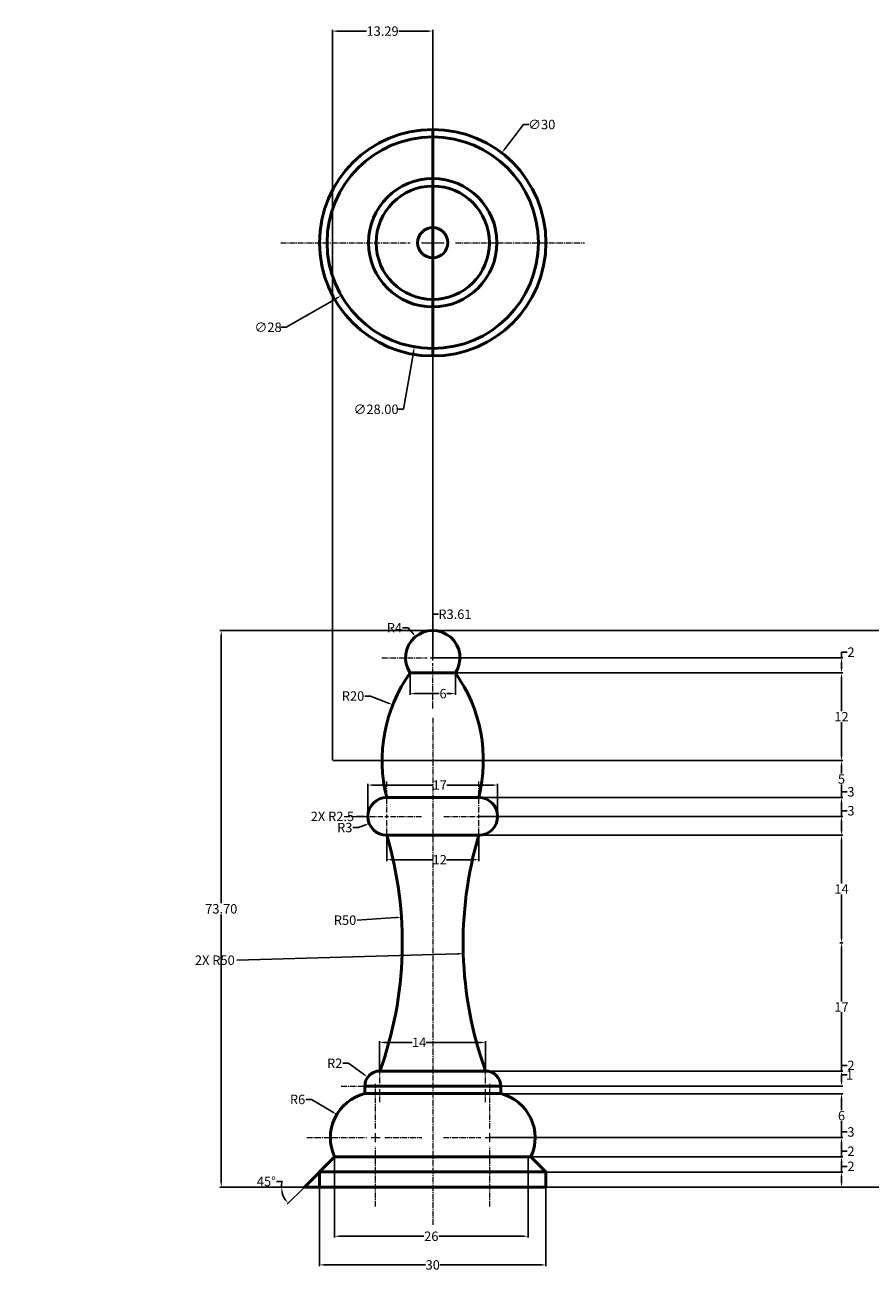
# Model space of a CAD drawing. Units: millimetres. Extents: x 184 to 390, y 95 to 263.
# Tile 1 of 2: x 184 to 296, y 98 to 263. Entities that reach past the tile are written whole.
import ezdxf

# ---------------------------------------------------------------- set-up
doc = ezdxf.new("R2010")
doc.units = ezdxf.units.MM
doc.header["$MEASUREMENT"] = 0
doc.linetypes.add('CENTER2', pattern=[1.125, 0.75, -0.125, 0.125, -0.125])
for name, color, linetype, lineweight in [('M-CNTR', 1, 'CENTER2', 18), ('M-DIMS', 2, 'Continuous', 25), ('M-OUTL', 7, 'Continuous', 50)]:
    doc.layers.add(name, color=color, linetype=linetype, lineweight=lineweight)
doc.styles.get("Standard").update_dxf_attribs({"font": 'arial.ttf'})
doc.dimstyles.get("Standard").update_dxf_attribs({"dimtxt": 1.25, "dimasz": 0.75, "dimexe": 0.18, "dimexo": 0.0625, "dimgap": 0.09, "dimtad": 0, "dimtih": 1, "dimtoh": 1, "dimdec": 0, "dimzin": 0, "dimdsep": 46, "dimtxsty": 'Standard', "dimcen": 0.09, "dimadec": 0, "dimazin": 0, "dimtfac": 1, "dimtdec": 0, "dimtofl": 0, "dimtmove": 0, "dimatfit": 3, "dimfxl": 1, "dimtolj": 1, "dimtzin": 0, "dimarcsym": 0})

# ---------------------------------------------------------------- blocks, each defined once
blk = doc.blocks.new('*D1')
at = {"layer": 'Defpoints', "color": 0, "transparency": 16777216}
for p in [(225.21, 112.98), (221.21, 108.98), (221.21, 108.98), (223.21, 108.98), (218.57, 107.46)]:
    blk.add_point(p, dxfattribs=at)
at = {"layer": 'M-DIMS', "color": 0, "lineweight": -2, "transparency": 16777216}
for p, q in [((218.26, 109.73), (217.51, 109.73)), ((221.15, 108.98), (217.99, 108.98)), ((221.16, 108.94), (218.93, 106.71))]:
    blk.add_line(p, q, dxfattribs=at)
for start, end in [(165.8396, 180), (194.1604, 210.8396)]:
    blk.add_arc((221.21, 108.98), 3.04, start, end, dxfattribs=at)
at = {"layer": 'M-DIMS', "color": 0, "transparency": 16777216}
for points in [[(218.13, 108.22), (218.38, 108.26), (218.17, 108.98)], [(218.69, 107.5), (218.5, 107.35), (219.06, 106.83)]]:
    blk.add_solid(points, dxfattribs=at)
at = {"layer": 'M-DIMS', "color": 0, "transparency": 16777216, "insert": (216.17, 109.73), "char_height": 1.25, "attachment_point": 5}
blk.add_mtext('\\A1;45°', dxfattribs=at)
blk = doc.blocks.new('*D2')
at = {"layer": 'Defpoints', "color": 0, "transparency": 16777216}
for p in [(247.35, 245.93), (229.07, 222.14)]:
    blk.add_point(p, dxfattribs=at)
at = {"layer": 'M-DIMS', "color": 0, "lineweight": -2, "transparency": 16777216}
for p, q in [((250.24, 249.69), (247.8, 246.53)), ((250.99, 249.69), (250.24, 249.69)), ((238.12, 234.04), (238.3, 234.04)), ((238.21, 233.95), (238.21, 234.13))]:
    blk.add_line(p, q, dxfattribs=at)
at = {"layer": 'M-DIMS', "color": 0, "transparency": 16777216}
blk.add_solid([(247.71, 246.6), (247.9, 246.45), (247.35, 245.93)], dxfattribs=at)
at = {"layer": 'M-DIMS', "color": 0, "transparency": 16777216, "insert": (252.65, 249.69), "char_height": 1.25, "attachment_point": 5}
blk.add_mtext('\\A1;∅30', dxfattribs=at)
blk = doc.blocks.new('*U3')
at = {"layer": 'M-CNTR', "color": 0, "transparency": 16777216}
for p, q in [((0, 3), (0, 20.12)), ((-20.12, 0), (-3, 0)), ((3, 0), (20.12, 0)), ((0, -20.12), (0, -3))]:
    blk.add_line(p, q, dxfattribs=at)
at = {"layer": 'M-CNTR', "color": 0, "linetype": 'Continuous', "transparency": 16777216}
for p, q in [((-1.5, 0), (1.5, 0)), ((0, -1.5), (0, 1.5))]:
    blk.add_line(p, q, dxfattribs=at)
blk = doc.blocks.new('*U4')
at = {"layer": 'M-CNTR', "color": 0, "transparency": 16777216}
for p, q in [((0, 0.72), (0, 8.73)), ((-6.73, 0), (-0.72, 0)), ((0.72, 0), (6.73, 0)), ((0, -6.73), (0, -0.72))]:
    blk.add_line(p, q, dxfattribs=at)
at = {"layer": 'M-CNTR', "color": 0, "linetype": 'Continuous', "transparency": 16777216}
for p, q in [((-0.36, 0), (0.36, 0)), ((0, -0.36), (0, 0.36))]:
    blk.add_line(p, q, dxfattribs=at)
blk = doc.blocks.new('*U5')
at = {"layer": 'M-CNTR', "color": 0, "transparency": 16777216}
for p, q in [((0, 0.5), (0, 4.62)), ((-5.62, 0), (-0.5, 0)), ((0.5, 0), (4.62, 0)), ((0, -4.62), (0, -0.5))]:
    blk.add_line(p, q, dxfattribs=at)
at = {"layer": 'M-CNTR', "color": 0, "linetype": 'Continuous', "transparency": 16777216}
for p, q in [((-0.25, 0), (0.25, 0)), ((0, -0.25), (0, 0.25))]:
    blk.add_line(p, q, dxfattribs=at)
blk = doc.blocks.new('*U6')
at = {"layer": 'M-CNTR', "color": 0, "transparency": 16777216}
for p, q in [((0, 0.5), (0, 4.62)), ((-4.62, 0), (-0.5, 0)), ((0.5, 0), (5.62, 0)), ((0, -4.62), (0, -0.5))]:
    blk.add_line(p, q, dxfattribs=at)
at = {"layer": 'M-CNTR', "color": 0, "linetype": 'Continuous', "transparency": 16777216}
for p, q in [((-0.25, 0), (0.25, 0)), ((0, -0.25), (0, 0.25))]:
    blk.add_line(p, q, dxfattribs=at)
blk = doc.blocks.new('*U7')
at = {"layer": 'M-CNTR', "color": 0, "transparency": 16777216}
for p, q in [((0, 1.2), (0, 7.12)), ((-9.12, 0), (-1.2, 0)), ((1.2, 0), (6.12, 0)), ((0, -9.12), (0, -1.2))]:
    blk.add_line(p, q, dxfattribs=at)
at = {"layer": 'M-CNTR', "color": 0, "linetype": 'Continuous', "transparency": 16777216}
for p, q in [((-0.6, 0), (0.6, 0)), ((0, -0.6), (0, 0.6))]:
    blk.add_line(p, q, dxfattribs=at)
blk = doc.blocks.new('*U8')
at = {"layer": 'M-CNTR', "color": 0, "transparency": 16777216}
for p, q in [((0, 1.2), (0, 7.12)), ((-6.12, 0), (-1.2, 0)), ((1.2, 0), (9.12, 0)), ((0, -9.12), (0, -1.2))]:
    blk.add_line(p, q, dxfattribs=at)
at = {"layer": 'M-CNTR', "color": 0, "linetype": 'Continuous', "transparency": 16777216}
for p, q in [((-0.6, 0), (0.6, 0)), ((0, -0.6), (0, 0.6))]:
    blk.add_line(p, q, dxfattribs=at)
blk = doc.blocks.new('*U9')
at = {"layer": 'M-CNTR', "color": 0, "transparency": 16777216}
for p, q in [((0, 0.4), (0, 4.12)), ((-2.12, 0), (-0.4, 0)), ((0.4, 0), (5.12, 0)), ((0, -2.12), (0, -0.4))]:
    blk.add_line(p, q, dxfattribs=at)
at = {"layer": 'M-CNTR', "color": 0, "linetype": 'Continuous', "transparency": 16777216}
for p, q in [((-0.2, 0), (0.2, 0)), ((0, -0.2), (0, 0.2))]:
    blk.add_line(p, q, dxfattribs=at)
blk = doc.blocks.new('*U10')
at = {"layer": 'M-CNTR', "color": 0, "transparency": 16777216}
for p, q in [((0, 0.4), (0, 4.12)), ((-5.12, 0), (-0.4, 0)), ((0.4, 0), (2.12, 0)), ((0, -2.12), (0, -0.4))]:
    blk.add_line(p, q, dxfattribs=at)
at = {"layer": 'M-CNTR', "color": 0, "linetype": 'Continuous', "transparency": 16777216}
for p, q in [((-0.2, 0), (0.2, 0)), ((0, -0.2), (0, 0.2))]:
    blk.add_line(p, q, dxfattribs=at)
blk = doc.blocks.new('*U11')
at = {"layer": 'M-CNTR', "color": 0, "transparency": 16777216}
blk.add_line((0, 61.12), (0, -6.12), dxfattribs=at)
blk = doc.blocks.new('*D12')
at = {"layer": 'Defpoints', "color": 0, "transparency": 16777216}
for p in [(235.93, 181.87), (238.21, 179.07)]:
    blk.add_point(p, dxfattribs=at)
at = {"layer": 'M-DIMS', "color": 0, "lineweight": -2, "transparency": 16777216}
for p, q in [((234.22, 183.05), (234.97, 183.05)), ((234.97, 183.05), (235.46, 182.45)), ((238.12, 179.07), (238.3, 179.07)), ((238.21, 178.98), (238.21, 179.16))]:
    blk.add_line(p, q, dxfattribs=at)
at = {"layer": 'M-DIMS', "color": 0, "transparency": 16777216}
blk.add_solid([(235.56, 182.53), (235.36, 182.38), (235.93, 181.87)], dxfattribs=at)
at = {"layer": 'M-DIMS', "color": 0, "transparency": 16777216, "insert": (233.13, 183.05), "char_height": 1.25, "attachment_point": 5}
blk.add_mtext('\\A1;R4', dxfattribs=at)
blk = doc.blocks.new('*D13')
at = {"layer": 'Defpoints', "color": 0, "transparency": 16777216}
for p in [(253.21, 110.98), (292.36, 110.98), (253.21, 108.98)]:
    blk.add_point(p, dxfattribs=at)
at = {"layer": 'M-DIMS', "color": 0, "lineweight": -2, "transparency": 16777216}
for p, q in [((253.27, 110.98), (292.54, 110.98)), ((292.36, 110.98), (292.36, 111.73)), ((292.36, 111.73), (293.11, 111.73)), ((253.27, 108.98), (292.54, 108.98)), ((292.36, 109.73), (292.36, 110.23))]:
    blk.add_line(p, q, dxfattribs=at)
at = {"layer": 'M-DIMS', "color": 0, "transparency": 16777216}
for points in [[(292.24, 110.23), (292.49, 110.23), (292.36, 110.98)], [(292.24, 109.73), (292.49, 109.73), (292.36, 108.98)]]:
    blk.add_solid(points, dxfattribs=at)
at = {"layer": 'M-DIMS', "color": 0, "transparency": 16777216, "insert": (293.62, 111.73), "char_height": 1.25, "attachment_point": 5}
blk.add_mtext('\\A1;2', dxfattribs=at)
blk = doc.blocks.new('*D14')
at = {"layer": 'Defpoints', "color": 0, "transparency": 16777216}
for p in [(251.21, 112.98), (292.36, 112.98), (253.21, 110.98)]:
    blk.add_point(p, dxfattribs=at)
at = {"layer": 'M-DIMS', "color": 0, "lineweight": -2, "transparency": 16777216}
for p, q in [((251.27, 112.98), (292.54, 112.98)), ((292.36, 112.98), (292.36, 113.73)), ((292.36, 113.73), (293.11, 113.73)), ((292.36, 111.73), (292.36, 112.23)), ((253.27, 110.98), (292.54, 110.98))]:
    blk.add_line(p, q, dxfattribs=at)
at = {"layer": 'M-DIMS', "color": 0, "transparency": 16777216}
for points in [[(292.24, 112.23), (292.49, 112.23), (292.36, 112.98)], [(292.24, 111.73), (292.49, 111.73), (292.36, 110.98)]]:
    blk.add_solid(points, dxfattribs=at)
at = {"layer": 'M-DIMS', "color": 0, "transparency": 16777216, "insert": (293.62, 113.73), "char_height": 1.25, "attachment_point": 5}
blk.add_mtext('\\A1;2', dxfattribs=at)
blk = doc.blocks.new('*D15')
at = {"layer": 'Defpoints', "color": 0, "transparency": 16777216}
for p in [(245.77, 115.53), (292.36, 115.53), (251.21, 112.98)]:
    blk.add_point(p, dxfattribs=at)
at = {"layer": 'M-DIMS', "color": 0, "lineweight": -2, "transparency": 16777216}
for p, q in [((245.84, 115.53), (292.54, 115.53)), ((292.36, 115.53), (292.36, 116.28)), ((292.36, 116.28), (293.11, 116.28)), ((292.36, 113.73), (292.36, 114.78)), ((251.27, 112.98), (292.54, 112.98))]:
    blk.add_line(p, q, dxfattribs=at)
at = {"layer": 'M-DIMS', "color": 0, "transparency": 16777216}
for points in [[(292.24, 114.78), (292.49, 114.78), (292.36, 115.53)], [(292.24, 113.73), (292.49, 113.73), (292.36, 112.98)]]:
    blk.add_solid(points, dxfattribs=at)
at = {"layer": 'M-DIMS', "color": 0, "transparency": 16777216, "insert": (293.61, 116.28), "char_height": 1.25, "attachment_point": 5}
blk.add_mtext('\\A1;3', dxfattribs=at)
blk = doc.blocks.new('*D16')
at = {"layer": 'Defpoints', "color": 0, "transparency": 16777216}
for p in [(247.21, 121.35), (292.36, 121.35), (245.77, 115.53)]:
    blk.add_point(p, dxfattribs=at)
at = {"layer": 'M-DIMS', "color": 0, "lineweight": -2, "transparency": 16777216}
for p, q in [((247.27, 121.35), (292.54, 121.35)), ((292.36, 120.6), (292.36, 119.17)), ((292.36, 116.28), (292.36, 117.71)), ((245.84, 115.53), (292.54, 115.53))]:
    blk.add_line(p, q, dxfattribs=at)
at = {"layer": 'M-DIMS', "color": 0, "transparency": 16777216}
for points in [[(292.24, 120.6), (292.49, 120.6), (292.36, 121.35)], [(292.24, 116.28), (292.49, 116.28), (292.36, 115.53)]]:
    blk.add_solid(points, dxfattribs=at)
at = {"layer": 'M-DIMS', "color": 0, "transparency": 16777216, "insert": (292.36, 118.44), "char_height": 1.25, "attachment_point": 5}
blk.add_mtext('\\A1;6', dxfattribs=at)
blk = doc.blocks.new('*D17')
at = {"layer": 'Defpoints', "color": 0, "transparency": 16777216}
for p in [(247.21, 122.35), (292.36, 122.35), (247.21, 121.35)]:
    blk.add_point(p, dxfattribs=at)
at = {"layer": 'M-DIMS', "color": 0, "lineweight": -2, "transparency": 16777216}
for p, q in [((292.36, 123.1), (292.36, 123.85)), ((292.36, 123.85), (293.11, 123.85)), ((247.27, 122.35), (292.54, 122.35)), ((247.27, 121.35), (292.54, 121.35)), ((292.36, 120.6), (292.36, 119.85))]:
    blk.add_line(p, q, dxfattribs=at)
at = {"layer": 'M-DIMS', "color": 0, "transparency": 16777216}
for points in [[(292.24, 123.1), (292.49, 123.1), (292.36, 122.35)], [(292.24, 120.6), (292.49, 120.6), (292.36, 121.35)]]:
    blk.add_solid(points, dxfattribs=at)
at = {"layer": 'M-DIMS', "color": 0, "transparency": 16777216, "insert": (293.43, 123.85), "char_height": 1.25, "attachment_point": 5}
blk.add_mtext('\\A1;1', dxfattribs=at)
blk = doc.blocks.new('*D18')
at = {"layer": 'Defpoints', "color": 0, "transparency": 16777216}
for p in [(245.21, 124.35), (292.36, 124.35), (247.21, 122.35)]:
    blk.add_point(p, dxfattribs=at)
at = {"layer": 'M-DIMS', "color": 0, "lineweight": -2, "transparency": 16777216}
for p, q in [((245.27, 124.35), (292.54, 124.35)), ((292.36, 124.35), (292.36, 125.1)), ((292.36, 125.1), (293.11, 125.1)), ((247.27, 122.35), (292.54, 122.35)), ((292.36, 123.1), (292.36, 123.6))]:
    blk.add_line(p, q, dxfattribs=at)
at = {"layer": 'M-DIMS', "color": 0, "transparency": 16777216}
for points in [[(292.24, 123.6), (292.49, 123.6), (292.36, 124.35)], [(292.24, 123.1), (292.49, 123.1), (292.36, 122.35)]]:
    blk.add_solid(points, dxfattribs=at)
at = {"layer": 'M-DIMS', "color": 0, "transparency": 16777216, "insert": (293.62, 125.1), "char_height": 1.25, "attachment_point": 5}
blk.add_mtext('\\A1;2', dxfattribs=at)
blk = doc.blocks.new('*D19')
at = {"layer": 'Defpoints', "color": 0, "transparency": 16777216}
for p in [(292.24, 141.33), (292.36, 141.33), (245.21, 124.35)]:
    blk.add_point(p, dxfattribs=at)
at = {"layer": 'M-DIMS', "color": 0, "lineweight": -2, "transparency": 16777216}
for p, q in [((292.3, 141.33), (292.54, 141.33)), ((292.36, 140.58), (292.36, 133.56)), ((292.36, 125.1), (292.36, 132.13)), ((245.27, 124.35), (292.54, 124.35))]:
    blk.add_line(p, q, dxfattribs=at)
at = {"layer": 'M-DIMS', "color": 0, "transparency": 16777216}
for points in [[(292.24, 140.58), (292.49, 140.58), (292.36, 141.33)], [(292.24, 125.1), (292.49, 125.1), (292.36, 124.35)]]:
    blk.add_solid(points, dxfattribs=at)
at = {"layer": 'M-DIMS', "color": 0, "transparency": 16777216, "insert": (292.36, 132.84), "char_height": 1.25, "attachment_point": 5}
blk.add_mtext('\\A1;17', dxfattribs=at)
blk = doc.blocks.new('*D20')
at = {"layer": 'Defpoints', "color": 0, "transparency": 16777216}
for p in [(244.31, 155.57), (292.36, 155.57), (292.24, 141.33)]:
    blk.add_point(p, dxfattribs=at)
at = {"layer": 'M-DIMS', "color": 0, "lineweight": -2, "transparency": 16777216}
for p, q in [((244.37, 155.57), (292.54, 155.57)), ((292.36, 154.82), (292.36, 149.17)), ((292.36, 142.08), (292.36, 147.74)), ((292.3, 141.33), (292.54, 141.33))]:
    blk.add_line(p, q, dxfattribs=at)
at = {"layer": 'M-DIMS', "color": 0, "transparency": 16777216}
for points in [[(292.24, 154.82), (292.49, 154.82), (292.36, 155.57)], [(292.24, 142.08), (292.49, 142.08), (292.36, 141.33)]]:
    blk.add_solid(points, dxfattribs=at)
at = {"layer": 'M-DIMS', "color": 0, "transparency": 16777216, "insert": (292.36, 148.45), "char_height": 1.25, "attachment_point": 5}
blk.add_mtext('\\A1;14', dxfattribs=at)
blk = doc.blocks.new('*D21')
at = {"layer": 'Defpoints', "color": 0, "transparency": 16777216}
for p in [(244.31, 158.07), (292.36, 158.07), (244.31, 155.57)]:
    blk.add_point(p, dxfattribs=at)
at = {"layer": 'M-DIMS', "color": 0, "lineweight": -2, "transparency": 16777216}
for p, q in [((292.36, 158.07), (292.36, 158.82)), ((292.36, 158.82), (293.11, 158.82)), ((244.37, 158.07), (292.54, 158.07)), ((292.36, 156.32), (292.36, 157.32)), ((244.37, 155.57), (292.54, 155.57))]:
    blk.add_line(p, q, dxfattribs=at)
at = {"layer": 'M-DIMS', "color": 0, "transparency": 16777216}
for points in [[(292.24, 157.32), (292.49, 157.32), (292.36, 158.07)], [(292.24, 156.32), (292.49, 156.32), (292.36, 155.57)]]:
    blk.add_solid(points, dxfattribs=at)
at = {"layer": 'M-DIMS', "color": 0, "transparency": 16777216, "insert": (293.61, 158.82), "char_height": 1.25, "attachment_point": 5}
blk.add_mtext('\\A1;3', dxfattribs=at)
blk = doc.blocks.new('*D22')
at = {"layer": 'Defpoints', "color": 0, "transparency": 16777216}
for p in [(244.31, 160.57), (292.36, 160.57), (244.31, 158.07)]:
    blk.add_point(p, dxfattribs=at)
at = {"layer": 'M-DIMS', "color": 0, "lineweight": -2, "transparency": 16777216}
for p, q in [((244.37, 160.57), (292.54, 160.57)), ((292.36, 160.57), (292.36, 161.32)), ((292.36, 161.32), (293.11, 161.32)), ((292.36, 158.82), (292.36, 159.82)), ((244.37, 158.07), (292.54, 158.07))]:
    blk.add_line(p, q, dxfattribs=at)
at = {"layer": 'M-DIMS', "color": 0, "transparency": 16777216}
for points in [[(292.24, 159.82), (292.49, 159.82), (292.36, 160.57)], [(292.24, 158.82), (292.49, 158.82), (292.36, 158.07)]]:
    blk.add_solid(points, dxfattribs=at)
at = {"layer": 'M-DIMS', "color": 0, "transparency": 16777216, "insert": (293.61, 161.32), "char_height": 1.25, "attachment_point": 5}
blk.add_mtext('\\A1;3', dxfattribs=at)
blk = doc.blocks.new('*D23')
at = {"layer": 'Defpoints', "color": 0, "transparency": 16777216}
for p in [(224.92, 165.47), (292.36, 165.47), (244.31, 160.57)]:
    blk.add_point(p, dxfattribs=at)
at = {"layer": 'M-DIMS', "color": 0, "lineweight": -2, "transparency": 16777216}
for p, q in [((224.98, 165.47), (292.54, 165.47)), ((292.36, 164.72), (292.36, 163.75)), ((292.36, 161.32), (292.36, 162.3)), ((244.37, 160.57), (292.54, 160.57))]:
    blk.add_line(p, q, dxfattribs=at)
at = {"layer": 'M-DIMS', "color": 0, "transparency": 16777216}
for points in [[(292.24, 164.72), (292.49, 164.72), (292.36, 165.47)], [(292.24, 161.32), (292.49, 161.32), (292.36, 160.57)]]:
    blk.add_solid(points, dxfattribs=at)
at = {"layer": 'M-DIMS', "color": 0, "transparency": 16777216, "insert": (292.36, 163.02), "char_height": 1.25, "attachment_point": 5}
blk.add_mtext('\\A1;5', dxfattribs=at)
blk = doc.blocks.new('*D24')
at = {"layer": 'Defpoints', "color": 0, "transparency": 16777216}
for p in [(241.21, 177.07), (292.36, 177.07), (224.92, 165.47)]:
    blk.add_point(p, dxfattribs=at)
at = {"layer": 'M-DIMS', "color": 0, "lineweight": -2, "transparency": 16777216}
for p, q in [((241.27, 177.07), (292.54, 177.07)), ((292.36, 176.32), (292.36, 171.99)), ((292.36, 166.22), (292.36, 170.56)), ((224.98, 165.47), (292.54, 165.47))]:
    blk.add_line(p, q, dxfattribs=at)
at = {"layer": 'M-DIMS', "color": 0, "transparency": 16777216}
for points in [[(292.24, 176.32), (292.49, 176.32), (292.36, 177.07)], [(292.24, 166.22), (292.49, 166.22), (292.36, 165.47)]]:
    blk.add_solid(points, dxfattribs=at)
at = {"layer": 'M-DIMS', "color": 0, "transparency": 16777216, "insert": (292.36, 171.27), "char_height": 1.25, "attachment_point": 5}
blk.add_mtext('\\A1;12', dxfattribs=at)
blk = doc.blocks.new('*D25')
at = {"layer": 'Defpoints', "color": 0, "transparency": 16777216}
for p in [(238.21, 179.07), (292.36, 179.07), (241.21, 177.07)]:
    blk.add_point(p, dxfattribs=at)
at = {"layer": 'M-DIMS', "color": 0, "lineweight": -2, "transparency": 16777216}
for p, q in [((238.27, 179.07), (292.54, 179.07)), ((292.36, 179.07), (292.36, 179.82)), ((292.36, 179.82), (293.11, 179.82)), ((292.36, 177.82), (292.36, 178.32)), ((241.27, 177.07), (292.54, 177.07))]:
    blk.add_line(p, q, dxfattribs=at)
at = {"layer": 'M-DIMS', "color": 0, "transparency": 16777216}
for points in [[(292.24, 178.32), (292.49, 178.32), (292.36, 179.07)], [(292.24, 177.82), (292.49, 177.82), (292.36, 177.07)]]:
    blk.add_solid(points, dxfattribs=at)
at = {"layer": 'M-DIMS', "color": 0, "transparency": 16777216, "insert": (293.62, 179.82), "char_height": 1.25, "attachment_point": 5}
blk.add_mtext('\\A1;2', dxfattribs=at)
blk = doc.blocks.new('*D26')
at = {"layer": 'Defpoints', "color": 0, "transparency": 16777216}
for p in [(229.79, 157.14), (232.11, 158.07)]:
    blk.add_point(p, dxfattribs=at)
at = {"layer": 'M-DIMS', "color": 0, "lineweight": -2, "transparency": 16777216}
for p, q in [((228.39, 156.59), (229.09, 156.87)), ((232.02, 158.07), (232.2, 158.07)), ((232.11, 157.98), (232.11, 158.16)), ((227.64, 156.59), (228.39, 156.59))]:
    blk.add_line(p, q, dxfattribs=at)
at = {"layer": 'M-DIMS', "color": 0, "transparency": 16777216}
blk.add_solid([(229.04, 156.98), (229.14, 156.75), (229.79, 157.14)], dxfattribs=at)
at = {"layer": 'M-DIMS', "color": 0, "transparency": 16777216, "insert": (226.55, 156.59), "char_height": 1.25, "attachment_point": 5}
blk.add_mtext('\\A1;R3', dxfattribs=at)
blk = doc.blocks.new('*D27')
at = {"layer": 'Defpoints', "color": 0, "transparency": 16777216}
for p in [(232.91, 172.85), (251.5, 165.47)]:
    blk.add_point(p, dxfattribs=at)
at = {"layer": 'M-DIMS', "color": 0, "lineweight": -2, "transparency": 16777216}
for p, q in [((229.23, 174.01), (229.98, 174.01)), ((229.98, 174.01), (232.21, 173.13)), ((251.41, 165.47), (251.59, 165.47)), ((251.5, 165.38), (251.5, 165.56))]:
    blk.add_line(p, q, dxfattribs=at)
at = {"layer": 'M-DIMS', "color": 0, "transparency": 16777216}
blk.add_solid([(232.26, 173.24), (232.17, 173.01), (232.91, 172.85)], dxfattribs=at)
at = {"layer": 'M-DIMS', "color": 0, "transparency": 16777216, "insert": (227.65, 174.01), "char_height": 1.25, "attachment_point": 5}
blk.add_mtext('\\A1;R20', dxfattribs=at)
blk = doc.blocks.new('*D28')
at = {"layer": 'Defpoints', "color": 0, "transparency": 16777216}
for p in [(234.06, 144.73), (184.18, 141.33)]:
    blk.add_point(p, dxfattribs=at)
at = {"layer": 'M-DIMS', "color": 0, "lineweight": -2, "transparency": 16777216}
blk.add_line((228.18, 144.33), (233.32, 144.68), dxfattribs=at)
at = {"layer": 'M-DIMS', "color": 0, "transparency": 16777216}
blk.add_solid([(233.31, 144.8), (233.32, 144.55), (234.06, 144.73)], dxfattribs=at)
at = {"layer": 'M-DIMS', "color": 0, "transparency": 16777216, "insert": (226.59, 144.33), "char_height": 1.25, "attachment_point": 5}
blk.add_mtext('\\A1;R50', dxfattribs=at)
blk = doc.blocks.new('*D29')
at = {"layer": 'Defpoints', "color": 0, "transparency": 16777216}
for p in [(229.59, 123.53), (231.21, 122.35)]:
    blk.add_point(p, dxfattribs=at)
at = {"layer": 'M-DIMS', "color": 0, "lineweight": -2, "transparency": 16777216}
for p, q in [((226.31, 125.38), (227.06, 125.38)), ((227.06, 125.38), (228.99, 123.98)), ((231.12, 122.35), (231.3, 122.35)), ((231.21, 122.26), (231.21, 122.44))]:
    blk.add_line(p, q, dxfattribs=at)
at = {"layer": 'M-DIMS', "color": 0, "transparency": 16777216}
blk.add_solid([(229.06, 124.08), (228.91, 123.87), (229.59, 123.53)], dxfattribs=at)
at = {"layer": 'M-DIMS', "color": 0, "transparency": 16777216, "insert": (225.22, 125.38), "char_height": 1.25, "attachment_point": 5}
blk.add_mtext('\\A1;R2', dxfattribs=at)
blk = doc.blocks.new('*D30')
at = {"layer": 'Defpoints', "color": 0, "transparency": 16777216}
for p in [(225.49, 118.6), (230.64, 115.53)]:
    blk.add_point(p, dxfattribs=at)
at = {"layer": 'M-DIMS', "color": 0, "lineweight": -2, "transparency": 16777216}
for p, q in [((221.4, 120.59), (222.15, 120.59)), ((222.15, 120.59), (224.84, 118.98)), ((230.55, 115.53), (230.73, 115.53)), ((230.64, 115.44), (230.64, 115.62))]:
    blk.add_line(p, q, dxfattribs=at)
at = {"layer": 'M-DIMS', "color": 0, "transparency": 16777216}
blk.add_solid([(224.91, 119.09), (224.78, 118.88), (225.49, 118.6)], dxfattribs=at)
at = {"layer": 'M-DIMS', "color": 0, "transparency": 16777216, "insert": (220.3, 120.59), "char_height": 1.25, "attachment_point": 5}
blk.add_mtext('\\A1;R6', dxfattribs=at)
blk = doc.blocks.new('*D31')
at = {"layer": 'Defpoints', "color": 0, "transparency": 16777216}
for p in [(223.21, 108.98), (253.21, 108.98), (253.21, 98.68)]:
    blk.add_point(p, dxfattribs=at)
at = {"layer": 'M-DIMS', "color": 0, "lineweight": -2, "transparency": 16777216}
for p, q in [((223.21, 108.92), (223.21, 98.5)), ((253.21, 108.92), (253.21, 98.5)), ((223.96, 98.68), (237.23, 98.68)), ((252.46, 98.68), (239.19, 98.68))]:
    blk.add_line(p, q, dxfattribs=at)
at = {"layer": 'M-DIMS', "color": 0, "transparency": 16777216}
for points in [[(223.96, 98.81), (223.96, 98.56), (223.21, 98.68)], [(252.46, 98.81), (252.46, 98.56), (253.21, 98.68)]]:
    blk.add_solid(points, dxfattribs=at)
at = {"layer": 'M-DIMS', "color": 0, "transparency": 16777216, "insert": (238.21, 98.68), "char_height": 1.25, "attachment_point": 5}
blk.add_mtext('\\A1;30', dxfattribs=at)
blk = doc.blocks.new('*D32')
at = {"layer": 'Defpoints', "color": 0, "transparency": 16777216}
for p in [(225.21, 112.98), (250.83, 112.98), (250.83, 102.47)]:
    blk.add_point(p, dxfattribs=at)
at = {"layer": 'M-DIMS', "color": 0, "lineweight": -2, "transparency": 16777216}
for p, q in [((225.21, 112.92), (225.21, 102.29)), ((250.83, 112.92), (250.83, 102.29)), ((225.96, 102.47), (237.02, 102.47)), ((250.08, 102.47), (239.01, 102.47))]:
    blk.add_line(p, q, dxfattribs=at)
at = {"layer": 'M-DIMS', "color": 0, "transparency": 16777216}
for points in [[(225.96, 102.6), (225.96, 102.35), (225.21, 102.47)], [(250.08, 102.6), (250.08, 102.35), (250.83, 102.47)]]:
    blk.add_solid(points, dxfattribs=at)
at = {"layer": 'M-DIMS', "color": 0, "transparency": 16777216, "insert": (238.02, 102.47), "char_height": 1.25, "attachment_point": 5}
blk.add_mtext('\\A1;26', dxfattribs=at)
blk = doc.blocks.new('*D33')
at = {"layer": 'Defpoints', "color": 0, "transparency": 16777216}
for p in [(232.11, 155.57), (244.31, 155.57), (244.31, 152.34)]:
    blk.add_point(p, dxfattribs=at)
at = {"layer": 'M-DIMS', "color": 0, "lineweight": -2, "transparency": 16777216}
for p, q in [((232.11, 155.51), (232.11, 152.16)), ((244.31, 155.51), (244.31, 152.16)), ((232.86, 152.34), (238.21, 152.34)), ((243.56, 152.34), (240.05, 152.34))]:
    blk.add_line(p, q, dxfattribs=at)
at = {"layer": 'M-DIMS', "color": 0, "transparency": 16777216}
for points in [[(232.86, 152.46), (232.86, 152.21), (232.11, 152.34)], [(243.56, 152.46), (243.56, 152.21), (244.31, 152.34)]]:
    blk.add_solid(points, dxfattribs=at)
at = {"layer": 'M-DIMS', "color": 0, "transparency": 16777216, "insert": (239.13, 152.34), "char_height": 1.25, "attachment_point": 5}
blk.add_mtext('\\A1;12', dxfattribs=at)
blk = doc.blocks.new('*D34')
at = {"layer": 'Defpoints', "color": 0, "transparency": 16777216}
for p in [(245.21, 128.14), (231.16, 124.35), (245.21, 124.35)]:
    blk.add_point(p, dxfattribs=at)
at = {"layer": 'M-DIMS', "color": 0, "lineweight": -2, "transparency": 16777216}
for p, q in [((231.16, 124.42), (231.16, 128.32)), ((231.91, 128.14), (235.49, 128.14)), ((244.46, 128.14), (237.34, 128.14)), ((245.21, 124.42), (245.21, 128.32))]:
    blk.add_line(p, q, dxfattribs=at)
at = {"layer": 'M-DIMS', "color": 0, "transparency": 16777216}
for points in [[(231.91, 128.26), (231.91, 128.01), (231.16, 128.14)], [(244.46, 128.26), (244.46, 128.01), (245.21, 128.14)]]:
    blk.add_solid(points, dxfattribs=at)
at = {"layer": 'M-DIMS', "color": 0, "transparency": 16777216, "insert": (236.41, 128.14), "char_height": 1.25, "attachment_point": 5}
blk.add_mtext('\\A1;14', dxfattribs=at)
blk = doc.blocks.new('*D35')
at = {"layer": 'Defpoints', "color": 0, "transparency": 16777216}
for p in [(235.21, 177.07), (241.21, 177.07), (241.21, 174.33)]:
    blk.add_point(p, dxfattribs=at)
at = {"layer": 'M-DIMS', "color": 0, "lineweight": -2, "transparency": 16777216}
for p, q in [((235.21, 177.01), (235.21, 174.15)), ((241.21, 177.01), (241.21, 174.15)), ((235.96, 174.33), (239.08, 174.33)), ((240.46, 174.33), (240.09, 174.33))]:
    blk.add_line(p, q, dxfattribs=at)
at = {"layer": 'M-DIMS', "color": 0, "transparency": 16777216}
for points in [[(235.96, 174.46), (235.96, 174.21), (235.21, 174.33)], [(240.46, 174.46), (240.46, 174.21), (241.21, 174.33)]]:
    blk.add_solid(points, dxfattribs=at)
at = {"layer": 'M-DIMS', "color": 0, "transparency": 16777216, "insert": (239.58, 174.33), "char_height": 1.25, "attachment_point": 5}
blk.add_mtext('\\A1;6', dxfattribs=at)
blk = doc.blocks.new('*D36')
at = {"layer": 'Defpoints', "color": 0, "transparency": 16777216}
for p in [(246.81, 162.22), (229.61, 158.07), (246.81, 158.07)]:
    blk.add_point(p, dxfattribs=at)
at = {"layer": 'M-DIMS', "color": 0, "lineweight": -2, "transparency": 16777216}
for p, q in [((229.61, 158.14), (229.61, 162.4)), ((230.36, 162.22), (238.21, 162.22)), ((246.06, 162.22), (240.06, 162.22)), ((246.81, 158.14), (246.81, 162.4))]:
    blk.add_line(p, q, dxfattribs=at)
at = {"layer": 'M-DIMS', "color": 0, "transparency": 16777216}
for points in [[(230.36, 162.34), (230.36, 162.09), (229.61, 162.22)], [(246.06, 162.34), (246.06, 162.09), (246.81, 162.22)]]:
    blk.add_solid(points, dxfattribs=at)
at = {"layer": 'M-DIMS', "color": 0, "transparency": 16777216, "insert": (239.13, 162.22), "char_height": 1.25, "attachment_point": 5}
blk.add_mtext('\\A1;17', dxfattribs=at)
blk = doc.blocks.new('*D37')
at = {"layer": 'Defpoints', "color": 0, "transparency": 16777216}
for p in [(238.21, 262.06), (238.21, 179.07), (224.92, 165.47)]:
    blk.add_point(p, dxfattribs=at)
at = {"layer": 'M-DIMS', "color": 0, "lineweight": -2, "transparency": 16777216}
for p, q in [((224.92, 165.53), (224.92, 262.24)), ((225.67, 262.06), (229.42, 262.06)), ((237.46, 262.06), (233.7, 262.06)), ((238.21, 179.14), (238.21, 262.24))]:
    blk.add_line(p, q, dxfattribs=at)
at = {"layer": 'M-DIMS', "color": 0, "transparency": 16777216}
for points in [[(225.67, 262.18), (225.67, 261.93), (224.92, 262.06)], [(237.46, 262.18), (237.46, 261.93), (238.21, 262.06)]]:
    blk.add_solid(points, dxfattribs=at)
at = {"layer": 'M-DIMS', "color": 0, "transparency": 16777216, "insert": (231.56, 262.06), "char_height": 1.25, "attachment_point": 5}
blk.add_mtext('\\A1;13.29', dxfattribs=at)
blk = doc.blocks.new('*D38')
at = {"layer": 'Defpoints', "color": 0, "transparency": 16777216}
for p in [(238.21, 182.68), (238.21, 179.07)]:
    blk.add_point(p, dxfattribs=at)
at = {"layer": 'M-DIMS', "color": 0, "lineweight": -2, "transparency": 16777216}
for p, q in [((238.96, 184.84), (238.21, 184.84)), ((238.21, 184.84), (238.21, 183.43)), ((238.12, 179.07), (238.3, 179.07)), ((238.21, 178.98), (238.21, 179.16))]:
    blk.add_line(p, q, dxfattribs=at)
at = {"layer": 'M-DIMS', "color": 0, "transparency": 16777216}
blk.add_solid([(238.08, 183.43), (238.33, 183.43), (238.21, 182.68)], dxfattribs=at)
at = {"layer": 'M-DIMS', "color": 0, "transparency": 16777216, "insert": (241.15, 184.84), "char_height": 1.25, "attachment_point": 5}
blk.add_mtext('\\A1;R3.61', dxfattribs=at)
blk = doc.blocks.new('*D39')
at = {"layer": 'Defpoints', "color": 0, "transparency": 16777216}
for p in [(229.61, 158.07), (232.11, 158.07)]:
    blk.add_point(p, dxfattribs=at)
at = {"layer": 'M-DIMS', "color": 0, "lineweight": -2, "transparency": 16777216}
for p, q in [((228.11, 158.07), (228.86, 158.07)), ((232.02, 158.07), (232.2, 158.07)), ((232.11, 157.98), (232.11, 158.16))]:
    blk.add_line(p, q, dxfattribs=at)
at = {"layer": 'M-DIMS', "color": 0, "transparency": 16777216}
blk.add_solid([(228.86, 158.2), (228.86, 157.95), (229.61, 158.07)], dxfattribs=at)
at = {"layer": 'M-DIMS', "color": 0, "transparency": 16777216, "insert": (224.92, 158.07), "char_height": 1.25, "attachment_point": 5}
blk.add_mtext('\\A1;2X R2.5', dxfattribs=at)
blk = doc.blocks.new('*D40')
at = {"layer": 'Defpoints', "color": 0, "transparency": 16777216}
for p in [(292.24, 141.33), (242.26, 139.89)]:
    blk.add_point(p, dxfattribs=at)
at = {"layer": 'M-DIMS', "color": 0, "lineweight": -2, "transparency": 16777216}
for p, q in [((292.15, 141.33), (292.33, 141.33)), ((292.24, 141.24), (292.24, 141.42)), ((212.27, 139.03), (241.51, 139.87))]:
    blk.add_line(p, q, dxfattribs=at)
at = {"layer": 'M-DIMS', "color": 0, "transparency": 16777216}
blk.add_solid([(241.5, 140), (241.51, 139.75), (242.26, 139.89)], dxfattribs=at)
at = {"layer": 'M-DIMS', "color": 0, "transparency": 16777216, "insert": (209.34, 139.03), "char_height": 1.25, "attachment_point": 5}
blk.add_mtext('\\A1;2X R50', dxfattribs=at)
blk = doc.blocks.new('*D41')
at = {"layer": 'Defpoints', "color": 0, "transparency": 16777216}
for p in [(250.33, 241.04), (226.08, 227.04)]:
    blk.add_point(p, dxfattribs=at)
at = {"layer": 'M-DIMS', "color": 0, "lineweight": -2, "transparency": 16777216}
for p, q in [((238.12, 234.04), (238.3, 234.04)), ((238.21, 233.95), (238.21, 234.13)), ((218.81, 222.84), (225.44, 226.66)), ((218.06, 222.84), (218.81, 222.84))]:
    blk.add_line(p, q, dxfattribs=at)
at = {"layer": 'M-DIMS', "color": 0, "transparency": 16777216}
blk.add_solid([(225.37, 226.77), (225.5, 226.55), (226.08, 227.04)], dxfattribs=at)
at = {"layer": 'M-DIMS', "color": 0, "transparency": 16777216, "insert": (216.39, 222.84), "char_height": 1.25, "attachment_point": 5}
blk.add_mtext('\\A1;∅28', dxfattribs=at)
blk = doc.blocks.new('*D53')
at = {"layer": 'Defpoints', "color": 0, "transparency": 16777216}
for p in [(210.19, 182.68), (336.1, 182.68), (321.1, 108.98)]:
    blk.add_point(p, dxfattribs=at)
at = {"layer": 'M-DIMS', "color": 0, "lineweight": -2, "transparency": 16777216}
for p, q in [((336.04, 182.68), (210.01, 182.68)), ((210.19, 181.93), (210.19, 146.56)), ((210.19, 109.73), (210.19, 145.1)), ((321.04, 108.98), (210.01, 108.98))]:
    blk.add_line(p, q, dxfattribs=at)
at = {"layer": 'M-DIMS', "color": 0, "transparency": 16777216}
for points in [[(210.06, 181.93), (210.31, 181.93), (210.19, 182.68)], [(210.06, 109.73), (210.31, 109.73), (210.19, 108.98)]]:
    blk.add_solid(points, dxfattribs=at)
at = {"layer": 'M-DIMS', "color": 0, "transparency": 16777216, "insert": (210.19, 145.83), "char_height": 1.25, "attachment_point": 5}
blk.add_mtext('\\A1;73.70', dxfattribs=at)
blk = doc.blocks.new('*D60')
at = {"layer": 'Defpoints', "color": 0, "transparency": 16777216}
for p in [(240.64, 247.83), (235.78, 220.25)]:
    blk.add_point(p, dxfattribs=at)
at = {"layer": 'M-DIMS', "color": 0, "lineweight": -2, "transparency": 16777216}
for p, q in [((238.12, 234.04), (238.3, 234.04)), ((238.21, 233.95), (238.21, 234.13)), ((234.32, 211.98), (235.65, 219.51)), ((233.57, 211.98), (234.32, 211.98))]:
    blk.add_line(p, q, dxfattribs=at)
at = {"layer": 'M-DIMS', "color": 0, "transparency": 16777216}
blk.add_solid([(235.53, 219.53), (235.77, 219.49), (235.78, 220.25)], dxfattribs=at)
at = {"layer": 'M-DIMS', "color": 0, "transparency": 16777216, "insert": (230.7, 211.98), "char_height": 1.25, "attachment_point": 5}
blk.add_mtext('\\A1;∅28.00', dxfattribs=at)

msp = doc.modelspace()

# ---------------------------------------------------------------- linework, layer by layer
at = {"layer": 'M-OUTL'}
for p, q in [((238.2079, 249.0386), (238.2079, 219.0386)), ((238.2079, 177.0741), (235.2079, 177.0741)), ((238.2079, 177.0741), (237.0741, 177.0741)), ((238.2079, 177.0741), (239.3418, 177.0741)), ((238.2079, 177.0741), (241.2079, 177.0741)), ((232.1079, 160.5741), (238.2079, 160.5741)), ((244.3079, 160.5741), (238.2079, 160.5741)), ((238.2079, 155.5741), (232.1079, 155.5741)), ((238.2079, 155.5741), (232.1079, 155.5741)), ((238.2079, 155.5741), (244.3079, 155.5741)), ((231.2079, 124.3541), (245.2079, 124.3541)), ((229.2079, 121.3541), (229.2079, 122.3541)), ((229.2079, 122.3541), (247.2079, 122.3541)), ((247.2079, 122.3541), (247.2079, 121.3541)), ((238.2079, 121.3541), (229.2079, 121.3541)), ((238.2079, 121.3541), (247.2079, 121.3541)), ((225.2079, 112.9841), (221.2079, 108.9841)), ((225.2079, 112.9841), (238.2079, 112.9841)), ((251.2079, 112.9841), (238.2079, 112.9841)), ((251.2079, 112.9841), (253.2079, 110.9841)), ((253.2079, 110.9841), (223.2079, 110.9841)), ((223.2079, 110.9841), (223.2079, 108.9841)), ((253.2079, 108.9841), (253.2079, 110.9841)), ((223.2079, 108.9841), (221.2079, 108.9841)), ((223.2079, 108.9841), (238.2079, 108.9841)), ((238.2079, 108.9841), (253.2079, 108.9841))]:
    msp.add_line(p, q, dxfattribs=at)
for radius in [15, 14, 8.5, 7.5, 2]:
    msp.add_circle((238.2079, 234.0386), radius, dxfattribs=at)
for centre, radius, start, end in [((238.2079, 179.0741), 3.6056, 326.309932, 213.690068), ((251.4989, 165.4722), 20, 144.542648, 194.176113), ((224.917, 165.4722), 20, 345.823887, 35.457352), ((232.1079, 158.0741), 2.5, 90, 270), ((244.3079, 158.0741), 2.5, 270, 90), ((184.179, 141.3328), 50, 340.149068, 16.548438), ((292.2369, 141.3328), 50, 163.451562, 199.850932), ((231.2079, 122.3541), 2, 90, 180), ((245.2079, 122.3541), 2, 0, 90), ((230.642, 115.528), 6, 103.827775, 205.086211), ((245.7739, 115.528), 6, 334.913789, 76.172225)]:
    msp.add_arc(centre, radius, start, end, dxfattribs=at)

# ---------------------------------------------------------------- block references
at = {"layer": 'M-CNTR'}
for name, p in [('*U3', (238.2079, 234.0386)), ('*U4', (238.2079, 179.0741)), ('*U11', (238.2079, 109.9841)), ('*U5', (232.1079, 158.0741)), ('*U6', (244.3079, 158.0741)), ('*U10', (231.2079, 122.3541)), ('*U9', (245.2079, 122.3541)), ('*U7', (230.642, 115.528)), ('*U8', (245.7739, 115.528))]:
    msp.add_blockref(name, p, dxfattribs=at)

# ---------------------------------------------------------------- dimensions: what is measured, and where the dimension line sits
at = {"layer": 'M-DIMS'}
for base, p1, p2, override, picture, middle in [((238.2079, 262.0586), (224.917, 165.4722), (238.2079, 179.0741), {"dimdec": 2, "dimlfac": 1, "dimrnd": 0, "dimzin": 0, "dimdsep": 46, "dimlunit": 2}, '*D37', (231.5625, 262.0586)), ((250.8278, 102.4714), (225.2079, 112.9841), (250.8278, 112.9841), {"dimclrd": 0, "dimclre": 0, "dimclrt": 0}, '*D32', (238.0179, 102.4714)), ((253.2079, 98.6812), (223.2079, 108.9841), (253.2079, 108.9841), {"dimclrd": 0, "dimclre": 0, "dimclrt": 0}, '*D31', (238.2079, 98.6812))]:
    dim = msp.add_linear_dim(base=base, p1=p1, p2=p2, dimstyle='Standard', override=override, dxfattribs=at)
    dim.commit()
    dim.dimension.update_dxf_attribs({"geometry": picture, "text_midpoint": middle})
for p1, p2, override, picture, middle in [((229.0682, 222.1448), (247.3477, 245.9325), {"dimclrd": 0, "dimclre": 0, "dimclrt": 0}, '*D2', (252.6512, 249.6938)), ((240.6357, 247.8265), (235.7801, 220.2508), {"dimdec": 2, "dimlfac": 1, "dimrnd": 0, "dimzin": 0, "dimdsep": 46, "dimlunit": 2}, '*D60', (230.6965, 211.978)), ((250.3313, 241.0404), (226.0846, 227.0369), {"dimdec": 0, "dimlfac": 1, "dimrnd": 0, "dimzin": 0, "dimdsep": 46, "dimlunit": 2}, '*D41', (216.394, 222.8358))]:
    dim = msp.add_diameter_dim_2p(p1=p1, p2=p2, dimstyle='Standard', override=override, dxfattribs=at)
    dim.commit()
    dim.dimension.update_dxf_attribs({"geometry": picture, "text_midpoint": middle, "dimtype": 163})
for center, mpoint, override, picture, middle in [((238.2079, 179.0741), (238.208, 182.6796), {"dimdec": 2, "dimlfac": 1, "dimrnd": 0, "dimzin": 0, "dimdsep": 46, "dimlunit": 2}, '*D38', (241.149, 184.843)), ((238.2079, 179.0741), (235.9338, 181.872), {"dimclrd": 0, "dimclre": 0, "dimclrt": 0}, '*D12', (233.1296, 183.0518)), ((251.4989, 165.4722), (232.9092, 172.8493), {"dimclrd": 0, "dimclre": 0, "dimclrt": 0}, '*D27', (227.6489, 174.0116)), ((184.179, 141.3328), (234.0634, 144.7299), {"dimclrd": 0, "dimclre": 0, "dimclrt": 0}, '*D28', (228.1755, 144.3289)), ((231.2079, 122.3541), (229.5923, 123.5329), {"dimclrd": 0, "dimclre": 0, "dimclrt": 0}, '*D29', (225.2167, 125.382)), ((230.642, 115.528), (225.4882, 118.6003), {"dimclrd": 0, "dimclre": 0, "dimclrt": 0}, '*D30', (220.3026, 120.5903))]:
    dim = msp.add_radius_dim(center=center, mpoint=mpoint, dimstyle='Standard', override=override, dxfattribs=at)
    dim.commit()
    dim.dimension.update_dxf_attribs({"geometry": picture, "text_midpoint": middle, "dimtype": 164})
for base, p1, p2, angle, override, picture, middle in [((210.1879, 182.6796), (321.101, 108.9841), (336.101, 182.6796), 90, {"dimdec": 2, "dimlfac": 1, "dimrnd": 0, "dimzin": 0, "dimdsep": 46, "dimlunit": 2}, '*D53', (210.1879, 145.8319)), ((292.3617, 179.0741), (241.2079, 177.0741), (238.2079, 179.0741), 270, {"dimclrd": 0, "dimclre": 0, "dimclrt": 0}, '*D25', (293.6156, 179.8241)), ((292.3617, 177.0741), (224.917, 165.4722), (241.2079, 177.0741), 270, {"dimclrd": 0, "dimclre": 0, "dimclrt": 0}, '*D24', (292.3617, 171.2731)), ((292.3617, 165.4722), (244.3079, 160.5741), (224.917, 165.4722), 270, {"dimclrd": 0, "dimclre": 0, "dimclrt": 0}, '*D23', (292.3617, 163.0231)), ((292.3616833556, 160.5740941605), (244.3079366142, 158.0740941604), (244.3079366142, 160.5740941605), 270, {"dimclrd": 0, "dimclre": 0, "dimclrt": 0}, '*D22', (293.6109602996, 161.3240941605)), ((292.3616833556, 158.0740941604), (244.3079366142, 155.5740941604), (244.3079366142, 158.0740941604), 270, {"dimclrd": 0, "dimclre": 0, "dimclrt": 0}, '*D21', (293.6109602996, 158.8240941604)), ((292.3617, 155.5741), (292.2369, 141.3328), (244.3079, 155.5741), 270, {"dimclrd": 0, "dimclre": 0, "dimclrt": 0}, '*D20', (292.3617, 148.4534)), ((292.3617, 141.3328), (245.2079, 124.3541), (292.2369, 141.3328), 270, {"dimclrd": 0, "dimclre": 0, "dimclrt": 0}, '*D19', (292.3617, 132.8434)), ((292.3617, 124.3541), (247.2079, 122.3541), (245.2079, 124.3541), 270, {"dimclrd": 0, "dimclre": 0, "dimclrt": 0}, '*D18', (293.6156, 125.1041)), ((292.3617, 122.3541), (247.2079, 121.3541), (247.2079, 122.3541), 270, {"dimclrd": 0, "dimclre": 0, "dimclrt": 0}, '*D17', (293.4319, 123.8541)), ((292.3617, 121.3541), (245.7739, 115.528), (247.2079, 121.3541), 270, {"dimclrd": 0, "dimclre": 0, "dimclrt": 0}, '*D16', (292.3617, 118.441)), ((292.3617, 115.528), (251.2079, 112.9841), (245.7739, 115.528), 270, {"dimclrd": 0, "dimclre": 0, "dimclrt": 0}, '*D15', (293.611, 116.278)), ((292.3617, 112.9841), (253.2079, 110.9841), (251.2079, 112.9841), 270, {"dimclrd": 0, "dimclre": 0, "dimclrt": 0}, '*D14', (293.6156, 113.7341)), ((292.3617, 110.9841), (253.2079, 108.9841), (253.2079, 110.9841), 270, {"dimclrd": 0, "dimclre": 0, "dimclrt": 0}, '*D13', (293.6156, 111.7341))]:
    dim = msp.add_linear_dim(base=base, p1=p1, p2=p2, angle=angle, dimstyle='Standard', override=override, dxfattribs=at)
    dim.commit()
    dim.dimension.update_dxf_attribs({"geometry": picture, "text_midpoint": middle})
for base, p1, p2, picture, middle in [((241.2079, 174.3331), (235.2079, 177.0741), (241.2079, 177.0741), '*D35', (239.5843, 174.3331)), ((246.8079, 162.2157), (229.6079, 158.0741), (246.8079, 158.0741), '*D36', (239.1344, 162.2157)), ((244.3079, 152.3388), (232.1079, 155.5741), (244.3079, 155.5741), '*D33', (239.128, 152.3388)), ((245.2079, 128.1358), (231.1553, 124.3541), (245.2079, 124.3541), '*D34', (236.4147, 128.1358))]:
    dim = msp.add_linear_dim(base=base, p1=p1, p2=p2, dimstyle='Standard', override={"dimclrd": 0, "dimclre": 0, "dimclrt": 0}, dxfattribs=at)
    dim.commit()
    dim.dimension.update_dxf_attribs({"geometry": picture, "text_midpoint": middle, "dimtype": 160})
for center, mpoint, override, picture, middle in [((232.1079, 158.0741), (229.6079, 158.074), {"dimdec": 1, "dimlfac": 1, "dimrnd": 0, "dimzin": 0, "dimdsep": 46, "dimlunit": 2}, '*D39', (228.1079, 158.0739)), ((292.2369, 141.3328), (242.2577, 139.892), {"dimdec": 0, "dimlfac": 1, "dimrnd": 0, "dimzin": 0, "dimdsep": 46, "dimlunit": 2}, '*D40', (212.2701, 139.0275))]:
    dim = msp.add_radius_dim(center=center, mpoint=mpoint, text='2X <>', dimstyle='Standard', override=override, dxfattribs=at)
    dim.commit()
    dim.dimension.update_dxf_attribs({"geometry": picture, "text_midpoint": middle, "dimtype": 164})
dim = msp.add_radius_dim(center=(232.1079, 158.0741), mpoint=(229.7873, 157.1443), dimstyle='Standard', override={"dimclrd": 0, "dimclre": 0, "dimclrt": 0}, dxfattribs=at)
dim.commit()
dim.dimension.update_dxf_attribs({"geometry": '*D26', "text_midpoint": (226.547, 156.5865)})
dim = msp.add_angular_dim_2l(base=(218.5732, 107.4629), line1=((223.2079, 108.9841), (221.2079, 108.9841)), line2=((225.2079, 112.9841), (221.2079, 108.9841)), dimstyle='Standard', override={"dimclrd": 0, "dimclre": 0, "dimclrt": 0}, dxfattribs=at)
dim.commit()
dim.dimension.update_dxf_attribs({"geometry": '*D1', "text_midpoint": (216.1667, 109.7284)})

doc.saveas('drawing.dxf')
